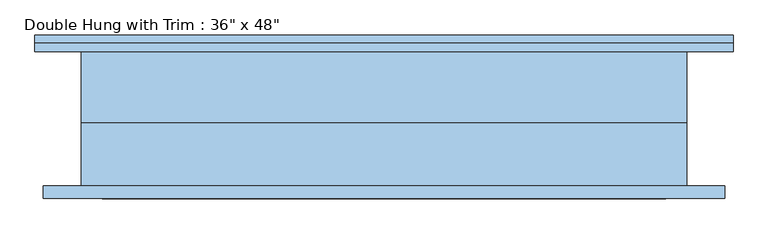
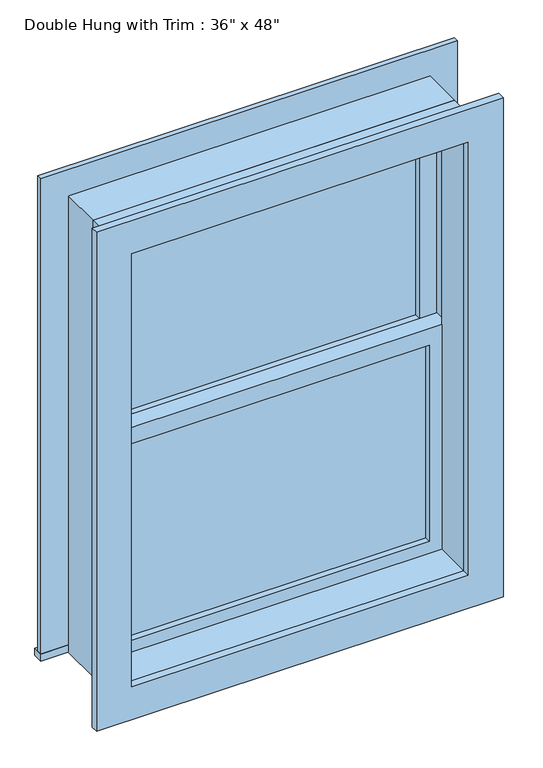
"""IFC4 building model written with IfcOpenShell, lengths in millimetres: window geometry."""

from ifc_helpers import new_model, si_unit, frame, origin, place, context, project, spatial, polyline, outline, extrude, source, transform, mapped, element, save


def window_31198920(model_context):
    return source(origin(), model_context, "Body", "SweptSolid", [
        extrude(outline(polyline([(-393.7, 22.225), (393.7, 22.225), (393.7, 9.525), (-393.7, 9.525), (-393.7, 22.225)])), frame((0.0, 0.0, 977.9), z_axis=(0.0, 0.0, 1.0), x_axis=(1.0, 0.0, 0.0)), (0.0, 0.0, 1.0), 523.875),
        extrude(outline(polyline([(1546.225, -438.15), (933.45, -438.15), (933.45, 438.15), (1546.225, 438.15), (1546.225, -438.15)]), holes=[polyline([(1501.775, -393.7), (1501.775, 393.7), (977.9, 393.7), (977.9, -393.7), (1501.775, -393.7)])]), frame((0.0, -6.35, 0.0), z_axis=(0.0, 1.0, 0.0), x_axis=(0.0, 0.0, 1.0)), (0.0, 0.0, 1.0), 44.45),
        extrude(outline(polyline([(-527.05, 127.0), (527.05, 127.0), (527.05, 101.6), (-527.05, 101.6), (-527.05, 127.0)])), frame((0.0, 0.0, 914.4), z_axis=(0.0, 0.0, 1.0), x_axis=(1.0, 0.0, 0.0)), (0.0, 0.0, 1.0), 19.05),
        extrude(outline(polyline([(2114.55, -438.15), (2114.55, 438.15), (933.45, 438.15), (933.45, 527.05), (2203.45, 527.05), (2203.45, -527.05), (933.45, -527.05), (933.45, -438.15), (2114.55, -438.15)])), frame((0.0, 101.6, 0.0), z_axis=(0.0, 1.0, 0.0), x_axis=(0.0, 0.0, 1.0)), (0.0, 0.0, 1.0), 12.7),
        extrude(outline(polyline([(2190.75, 514.35), (2190.75, -514.35), (857.25, -514.35), (857.25, 514.35), (2190.75, 514.35)]), holes=[polyline([(2101.85, 425.45), (946.15, 425.45), (946.15, -425.45), (2101.85, -425.45), (2101.85, 425.45)])]), frame((0.0, -120.65, 0.0), z_axis=(0.0, 1.0, 0.0), x_axis=(0.0, 0.0, 1.0)), (0.0, 0.0, 1.0), 19.05),
        extrude(outline(polyline([(393.7, 53.975), (-393.7, 53.975), (-393.7, 66.675), (393.7, 66.675), (393.7, 53.975)])), frame((0.0, 0.0, 1546.225), z_axis=(0.0, 0.0, 1.0), x_axis=(1.0, 0.0, 0.0)), (0.0, 0.0, 1.0), 523.875),
        extrude(outline(polyline([(2114.55, -438.15), (1501.775, -438.15), (1501.775, 438.15), (2114.55, 438.15), (2114.55, -438.15)]), holes=[polyline([(2070.1, -393.7), (2070.1, 393.7), (1546.225, 393.7), (1546.225, -393.7), (2070.1, -393.7)])]), frame((0.0, 38.1, 0.0), z_axis=(0.0, 1.0, 0.0), x_axis=(0.0, 0.0, 1.0)), (0.0, 0.0, 1.0), 44.45),
        extrude(outline(polyline([(2133.6, -457.2), (914.4, -457.2), (914.4, 457.2), (2133.6, 457.2), (2133.6, -457.2)]), holes=[polyline([(2101.85, -425.45), (2101.85, 425.45), (946.15, 425.45), (946.15, -425.45), (2101.85, -425.45)])]), frame((0.0, -101.6, 0.0), z_axis=(0.0, 1.0, 0.0), x_axis=(0.0, 0.0, 1.0)), (0.0, 0.0, 1.0), 95.25),
        extrude(outline(polyline([(2133.6, 457.2), (2133.6, -457.2), (914.4, -457.2), (914.4, 457.2), (2133.6, 457.2)]), holes=[polyline([(2114.55, 438.15), (933.45, 438.15), (933.45, -438.15), (2114.55, -438.15), (2114.55, 438.15)])]), frame((0.0, -6.35, 0.0), z_axis=(0.0, 1.0, 0.0), x_axis=(0.0, 0.0, 1.0)), (0.0, 0.0, 1.0), 107.95),
    ])


if __name__ == "__main__":
    model = new_model("IFC4")
    model_context = context("Model", 3, world=origin())
    ifc_project = project(units=[si_unit("LENGTHUNIT", "METRE", prefix="MILLI")], contexts=[model_context])
    site = spatial("IfcSite", under=ifc_project)
    building = spatial("IfcBuilding", under=site)
    placement = place(None, origin())
    window_shape = window_31198920(model_context)
    element("IfcWindow", 1, ObjectType="Double Hung with Trim : 36\" x 48\"", at=placement, inside=building, context=model_context, shape_type="MappedRepresentation", body=[
        mapped(window_shape, transform((0.0, 0.0, 0.0), x_axis=(1.0, 0.0, 0.0), y_axis=(0.0, 1.0, 0.0), z_axis=(0.0, 0.0, 1.0))),
    ])
    save(model, "model.ifc")

# Revit data of these elements
# Type "Double Hung with Trim : 36\" x 48\""
#   Type Mark = "13"
#   Construction Type Id = "GSP4R"
#   Assembly Code = "B2020100"
#   Analytic Construction = "1/8 in Pilkington single glazing"
#   Visual Light Transmittance = 0.9
#   Solar Heat Gain Coefficient = 0.78
#   Heat Transfer Coefficient (U) = 0.6496 BTU/(h·ft²·°F)
#   Height = 4' - 0"
#   Default Sill Height = 3' - 0"
#   Trim Projection - Ext. = 0' - 0 1/2"
#   Trim Projection - Int. = 0' - 0 3/4"
#   Trim Width - Exterior = 0' - 3 1/2"
#   Trim Width - Interior = 0' - 3 1/2"
#   Width = 3' - 0"
#   Window Inset = 0' - 0 3/4"
#   Define Thermal Properties by = 1
#   Glass Pane Material = Glass
#   Sash Material = Sash
#   Trim Exterior Material = Trim
#   Trim Interior Material = Trim
#   Wall Closure = (empty or 0)
# Element 1 (IfcWindow, "Double Hung with Trim : 36\" x 48\"")
#   Materials on its faces: "Sash", "Trim", "Glass"
# Materials
#   "Glass": class "Glass", colour RGB 0 128 192, transparency 0.75, Description = "Soda Lime Glass", Cost = 0
#   "Sash": class "Wood", colour RGB 224 178 126, transparency 0
#   "Trim": class "Wood", colour RGB 224 178 126, transparency 0
